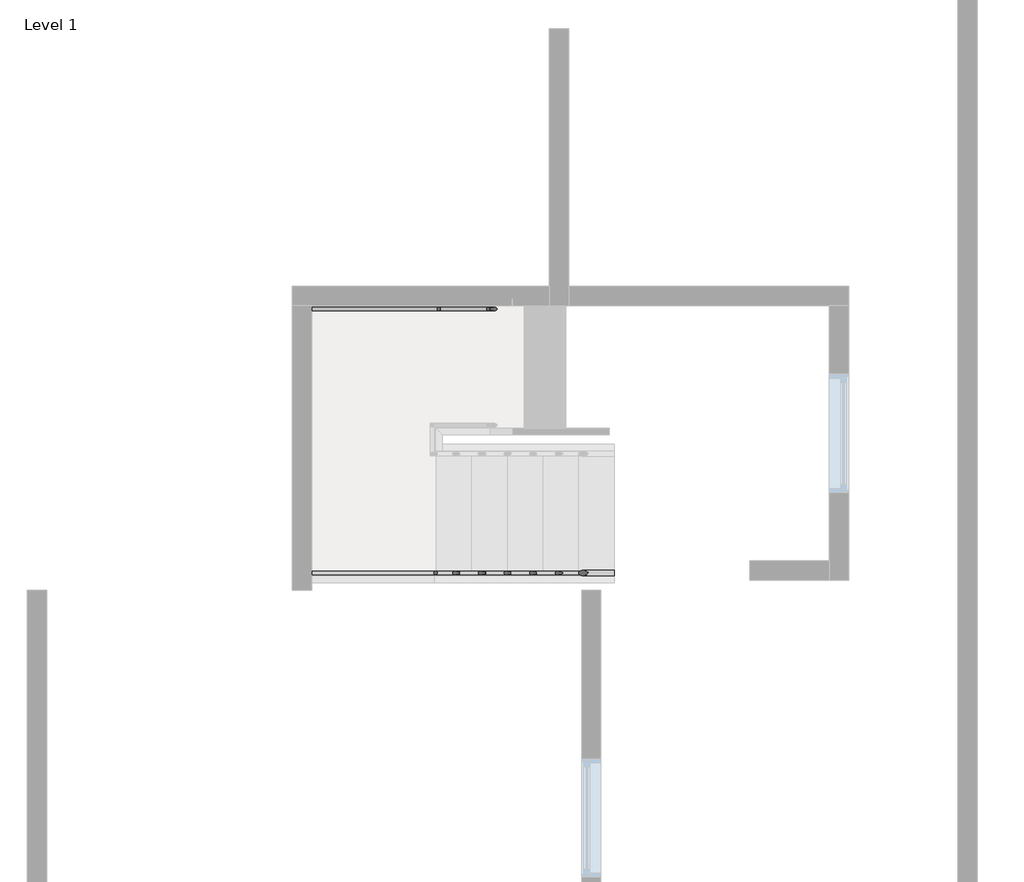
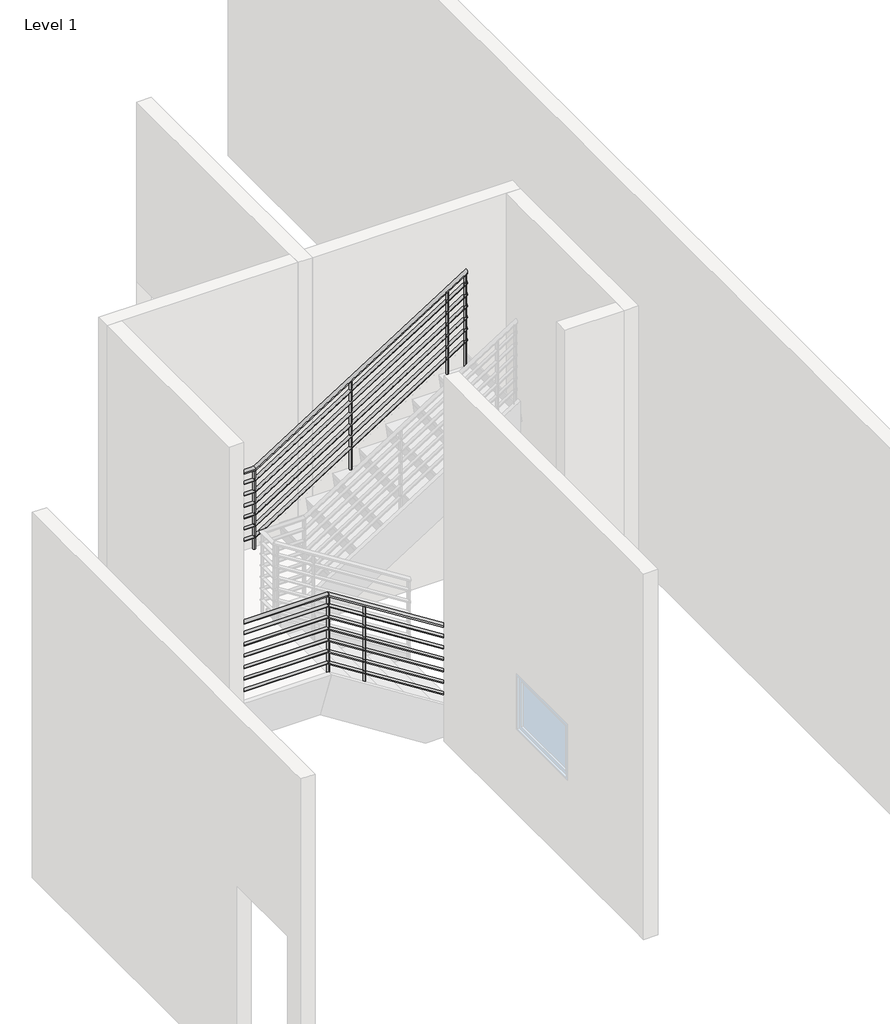
# One storey, part 2 of 4: 1 railing.
"""IFC4 building model written with IfcOpenShell, lengths in millimetres."""

from ifc_helpers import new_model, si_unit, point, frame, frame_2d, origin, place, context, project, spatial, circle_curve, ellipse_curve, trimmed, segment, composite_curve, outline, extrude, element, save
from ifc_brep_helpers import plane_surface, cylinder_surface, advanced_brep

model = new_model("IFC4")

# Units and contexts
model_context = context("Model", 3, world=origin())
ifc_project = project(units=[si_unit("LENGTHUNIT", "METRE", prefix="MILLI")], contexts=[model_context])

# Site, building, storey
site = spatial("IfcSite", under=ifc_project)
building = spatial("IfcBuilding", under=site)
storey = spatial("IfcBuildingStorey", under=building, Name="Level 1", Elevation=0.0)

# Railing
placement = place(None, origin())
element("IfcRailing", 1, ObjectType="900mm Pipe", at=placement, inside=storey, context=model_context, shape_type="SolidModel", body=[
    advanced_brep(
    [(-539.0915237, 888.4180557, 1050.2491997), (-539.0915237, 848.4180557, 1050.2491997), (-1919.8849767, 888.4180557, 1923.4782609), (-1919.8849767, 848.4180557, 1923.4782609), (-2868.717305, 888.4180557, 1923.4782609), (-2908.717305, 848.4180557, 1923.4782609), (-2868.717305, 2880.8309464, 1923.4782609), (-2908.717305, 2920.8309464, 1923.4782609), (-1501.6762623, 2880.8309464, 1923.4782609), (-1501.6762623, 2920.8309464, 1923.4782609), (692.5302847, 2880.8309464, 3311.1187649), (692.5302847, 2920.8309464, 3311.1187649)],
    [
        (0, 1, ellipse_curve(frame((-539.0915237, 868.4180557, 1050.2491997), z_axis=(1.0, 0.0, 0.0), x_axis=(0.0, 0.0, -1.0)), 23.6638438, 20.0)),
        (1, 0, ellipse_curve(frame((-539.0915237, 868.4180557, 1050.2491997), z_axis=(1.0, 0.0, 0.0), x_axis=(0.0, 0.0, -1.0)), 23.6638438, 20.0)),
        (0, 2),
        (2, 3, ellipse_curve(frame((-1919.8849767, 868.4180557, 1923.4782609), z_axis=(0.9605132043335073, 0.0, -0.2782344053149754), x_axis=(-0.278234405314975, 0.0, -0.9605132043335074)), 20.822202, 20.0)),
        (3, 1),
        (3, 2, ellipse_curve(frame((-1919.8849767, 868.4180557, 1923.4782609), z_axis=(0.9605132043335073, 0.0, -0.2782344053149754), x_axis=(-0.278234405314975, 0.0, -0.9605132043335074)), 20.822202, 20.0)),
        (2, 4),
        (4, 5, ellipse_curve(frame((-2888.717305, 868.4180557, 1923.4782609), z_axis=(0.7071067811865449, -0.7071067811865501, 0.0), x_axis=(0.7071067811865501, 0.7071067811865448, 0.0)), 28.2842712, 20.0)),
        (5, 3),
        (5, 4, ellipse_curve(frame((-2888.717305, 868.4180557, 1923.4782609), z_axis=(0.7071067811865449, -0.7071067811865501, 0.0), x_axis=(0.7071067811865501, 0.7071067811865448, 0.0)), 28.2842712, 20.0)),
        (4, 6),
        (6, 7, ellipse_curve(frame((-2888.717305, 2900.8309464, 1923.4782609), z_axis=(-0.7071067811865501, -0.7071067811865449, 0.0), x_axis=(0.7071067811865448, -0.7071067811865501, 0.0)), 28.2842712, 20.0)),
        (7, 5),
        (7, 6, ellipse_curve(frame((-2888.717305, 2900.8309464, 1923.4782609), z_axis=(-0.7071067811865501, -0.7071067811865449, 0.0), x_axis=(0.7071067811865448, -0.7071067811865501, 0.0)), 28.2842712, 20.0)),
        (6, 8),
        (8, 9, ellipse_curve(frame((-1501.6762623, 2900.8309464, 1923.4782609), z_axis=(-0.9605132043335073, 0.0, -0.27823440531497556), x_axis=(-0.2782344053149757, 0.0, 0.9605132043335073)), 20.822202, 20.0)),
        (9, 7),
        (9, 8, ellipse_curve(frame((-1501.6762623, 2900.8309464, 1923.4782609), z_axis=(-0.9605132043335073, 0.0, -0.27823440531497556), x_axis=(-0.2782344053149757, 0.0, 0.9605132043335073)), 20.822202, 20.0)),
        (10, 11, ellipse_curve(frame((692.5302847, 2900.8309464, 3311.1187649), z_axis=(1.0, 0.0, 0.0), x_axis=(0.0, 0.0, -1.0)), 23.6638438, 20.0)),
        (11, 10, ellipse_curve(frame((692.5302847, 2900.8309464, 3311.1187649), z_axis=(1.0, 0.0, 0.0), x_axis=(0.0, 0.0, -1.0)), 23.6638438, 20.0)),
        (8, 10),
        (11, 9),
    ],
    [
        plane_surface(frame((-539.0915237, 868.4180557, 1073.9130435), z_axis=(1.0, 0.0, 0.0), x_axis=(0.0, -1.0, 0.0))),
        cylinder_surface(frame((-549.7814365, 868.4180557, 1057.0096189), z_axis=(0.845171231398044, 0.0, -0.5344956404098298), x_axis=(0.0, -1.0, 0.0)), 20.0),
        cylinder_surface(frame((-1914.0915237, 868.4180557, 1923.4782609), z_axis=(1.0, 0.0, 0.0), x_axis=(0.0, -1.0, 0.0)), 20.0),
        cylinder_surface(frame((-2888.717305, 868.4180557, 1923.4782609), z_axis=(0.0, -1.0, 0.0), x_axis=(-1.0, 0.0, 0.0)), 20.0),
        cylinder_surface(frame((-2888.717305, 2900.8309464, 1923.4782609), z_axis=(-1.0, 0.0, 0.0), x_axis=(0.0, 1.0, 0.0)), 20.0),
        plane_surface(frame((692.5302847, 2900.8309464, 3334.7826087), z_axis=(1.0, 0.0, 0.0), x_axis=(0.0, 1.0, 0.0))),
        cylinder_surface(frame((-1496.7798025, 2900.8309464, 1926.5748362), z_axis=(-0.8451712313980438, 0.0, -0.5344956404098301), x_axis=(0.0, 1.0, 0.0)), 20.0),
    ],
    [
        (0, [[1, 2]]),
        (1, [[-1, 3, 4, 5]]),
        (1, [[-2, -5, 6, -3]]),
        (2, [[-4, 7, 8, 9]]),
        (2, [[-6, -9, 10, -7]]),
        (3, [[-8, 11, 12, 13]]),
        (3, [[-10, -13, 14, -11]]),
        (4, [[-12, 15, 16, 17]]),
        (4, [[-14, -17, 18, -15]]),
        (5, [[19, 20]]),
        (6, [[-16, 21, -20, 22]]),
        (6, [[-18, -22, -19, -21]]),
    ],
),
    advanced_brep(
    [(-539.0915237, 883.4180557, 931.1651606), (-539.0915237, 853.4180557, 931.1651606), (-1918.4366135, 883.4180557, 1803.4782609), (-1918.4366135, 853.4180557, 1803.4782609), (-2873.717305, 883.4180557, 1803.4782609), (-2903.717305, 853.4180557, 1803.4782609), (-2873.717305, 2885.8309464, 1803.4782609), (-2903.717305, 2915.8309464, 1803.4782609), (-1503.1246256, 2885.8309464, 1803.4782609), (-1503.1246256, 2915.8309464, 1803.4782609), (692.5302847, 2885.8309464, 3192.0347258), (692.5302847, 2915.8309464, 3192.0347258)],
    [
        (0, 1, ellipse_curve(frame((-539.0915237, 868.4180557, 931.1651606), z_axis=(1.0, 0.0, 0.0), x_axis=(0.0, 0.0, -1.0)), 17.7478828, 15.0)),
        (1, 0, ellipse_curve(frame((-539.0915237, 868.4180557, 931.1651606), z_axis=(1.0, 0.0, 0.0), x_axis=(0.0, 0.0, -1.0)), 17.7478828, 15.0)),
        (0, 2),
        (2, 3, ellipse_curve(frame((-1918.4366135, 868.4180557, 1803.4782609), z_axis=(0.9605132043335073, 0.0, -0.27823440531497545), x_axis=(-0.2782344053149749, 0.0, -0.9605132043335074)), 15.6166515, 15.0)),
        (3, 1),
        (3, 2, ellipse_curve(frame((-1918.4366135, 868.4180557, 1803.4782609), z_axis=(0.9605132043335073, 0.0, -0.27823440531497545), x_axis=(-0.2782344053149749, 0.0, -0.9605132043335074)), 15.6166515, 15.0)),
        (2, 4),
        (4, 5, ellipse_curve(frame((-2888.717305, 868.4180557, 1803.4782609), z_axis=(0.7071067811865449, -0.7071067811865501, 0.0), x_axis=(0.7071067811865501, 0.7071067811865448, 0.0)), 21.2132034, 15.0)),
        (5, 3),
        (5, 4, ellipse_curve(frame((-2888.717305, 868.4180557, 1803.4782609), z_axis=(0.7071067811865449, -0.7071067811865501, 0.0), x_axis=(0.7071067811865501, 0.7071067811865448, 0.0)), 21.2132034, 15.0)),
        (4, 6),
        (6, 7, ellipse_curve(frame((-2888.717305, 2900.8309464, 1803.4782609), z_axis=(-0.7071067811865501, -0.7071067811865449, 0.0), x_axis=(0.7071067811865448, -0.7071067811865501, 0.0)), 21.2132034, 15.0)),
        (7, 5),
        (7, 6, ellipse_curve(frame((-2888.717305, 2900.8309464, 1803.4782609), z_axis=(-0.7071067811865501, -0.7071067811865449, 0.0), x_axis=(0.7071067811865448, -0.7071067811865501, 0.0)), 21.2132034, 15.0)),
        (6, 8),
        (8, 9, ellipse_curve(frame((-1503.1246256, 2900.8309464, 1803.4782609), z_axis=(-0.9605132043335072, 0.0, -0.27823440531497556), x_axis=(-0.2782344053149761, 0.0, 0.9605132043335072)), 15.6166515, 15.0)),
        (9, 7),
        (9, 8, ellipse_curve(frame((-1503.1246256, 2900.8309464, 1803.4782609), z_axis=(-0.9605132043335072, 0.0, -0.27823440531497556), x_axis=(-0.2782344053149761, 0.0, 0.9605132043335072)), 15.6166515, 15.0)),
        (10, 11, ellipse_curve(frame((692.5302847, 2900.8309464, 3192.0347258), z_axis=(1.0, 0.0, 0.0), x_axis=(0.0, 0.0, -1.0)), 17.7478828, 15.0)),
        (11, 10, ellipse_curve(frame((692.5302847, 2900.8309464, 3192.0347258), z_axis=(1.0, 0.0, 0.0), x_axis=(0.0, 0.0, -1.0)), 17.7478828, 15.0)),
        (8, 10),
        (11, 9),
    ],
    [
        plane_surface(frame((-539.0915237, 868.4180557, 948.9130435), z_axis=(1.0, 0.0, 0.0), x_axis=(0.0, -1.0, 0.0))),
        cylinder_surface(frame((-547.1089583, 868.4180557, 936.235475), z_axis=(0.845171231398044, 0.0, -0.5344956404098299), x_axis=(0.0, -1.0, 0.0)), 15.0),
        cylinder_surface(frame((-1914.0915237, 868.4180557, 1803.4782609), z_axis=(1.0, 0.0, 0.0), x_axis=(0.0, -1.0, 0.0)), 15.0),
        cylinder_surface(frame((-2888.717305, 868.4180557, 1803.4782609), z_axis=(0.0, -1.0, 0.0), x_axis=(-1.0, 0.0, 0.0)), 15.0),
        cylinder_surface(frame((-2888.717305, 2900.8309464, 1803.4782609), z_axis=(-1.0, 0.0, 0.0), x_axis=(0.0, 1.0, 0.0)), 15.0),
        plane_surface(frame((692.5302847, 2900.8309464, 3209.7826087), z_axis=(1.0, 0.0, 0.0), x_axis=(0.0, 1.0, 0.0))),
        cylinder_surface(frame((-1499.4522807, 2900.8309464, 1805.8006924), z_axis=(-0.8451712313980437, 0.0, -0.5344956404098301), x_axis=(0.0, 1.0, 0.0)), 15.0),
    ],
    [
        (0, [[1, 2]]),
        (1, [[-1, 3, 4, 5]]),
        (1, [[-2, -5, 6, -3]]),
        (2, [[-4, 7, 8, 9]]),
        (2, [[-6, -9, 10, -7]]),
        (3, [[-8, 11, 12, 13]]),
        (3, [[-10, -13, 14, -11]]),
        (4, [[-12, 15, 16, 17]]),
        (4, [[-14, -17, 18, -15]]),
        (5, [[19, 20]]),
        (6, [[-16, 21, -20, 22]]),
        (6, [[-18, -22, -19, -21]]),
    ],
),
    advanced_brep(
    [(-539.0915237, 883.4180557, 806.1651606), (-539.0915237, 853.4180557, 806.1651606), (-1918.4366135, 883.4180557, 1678.4782609), (-1918.4366135, 853.4180557, 1678.4782609), (-2873.717305, 883.4180557, 1678.4782609), (-2903.717305, 853.4180557, 1678.4782609), (-2873.717305, 2885.8309464, 1678.4782609), (-2903.717305, 2915.8309464, 1678.4782609), (-1503.1246256, 2885.8309464, 1678.4782609), (-1503.1246256, 2915.8309464, 1678.4782609), (692.5302847, 2885.8309464, 3067.0347258), (692.5302847, 2915.8309464, 3067.0347258)],
    [
        (0, 1, ellipse_curve(frame((-539.0915237, 868.4180557, 806.1651606), z_axis=(1.0, 0.0, 0.0), x_axis=(0.0, 0.0, -1.0)), 17.7478828, 15.0)),
        (1, 0, ellipse_curve(frame((-539.0915237, 868.4180557, 806.1651606), z_axis=(1.0, 0.0, 0.0), x_axis=(0.0, 0.0, -1.0)), 17.7478828, 15.0)),
        (0, 2),
        (2, 3, ellipse_curve(frame((-1918.4366135, 868.4180557, 1678.4782609), z_axis=(0.9605132043335073, 0.0, -0.27823440531497545), x_axis=(-0.2782344053149749, 0.0, -0.9605132043335074)), 15.6166515, 15.0)),
        (3, 1),
        (3, 2, ellipse_curve(frame((-1918.4366135, 868.4180557, 1678.4782609), z_axis=(0.9605132043335073, 0.0, -0.27823440531497545), x_axis=(-0.2782344053149749, 0.0, -0.9605132043335074)), 15.6166515, 15.0)),
        (2, 4),
        (4, 5, ellipse_curve(frame((-2888.717305, 868.4180557, 1678.4782609), z_axis=(0.7071067811865449, -0.7071067811865501, 0.0), x_axis=(0.7071067811865501, 0.7071067811865448, 0.0)), 21.2132034, 15.0)),
        (5, 3),
        (5, 4, ellipse_curve(frame((-2888.717305, 868.4180557, 1678.4782609), z_axis=(0.7071067811865449, -0.7071067811865501, 0.0), x_axis=(0.7071067811865501, 0.7071067811865448, 0.0)), 21.2132034, 15.0)),
        (4, 6),
        (6, 7, ellipse_curve(frame((-2888.717305, 2900.8309464, 1678.4782609), z_axis=(-0.7071067811865501, -0.7071067811865449, 0.0), x_axis=(0.7071067811865448, -0.7071067811865501, 0.0)), 21.2132034, 15.0)),
        (7, 5),
        (7, 6, ellipse_curve(frame((-2888.717305, 2900.8309464, 1678.4782609), z_axis=(-0.7071067811865501, -0.7071067811865449, 0.0), x_axis=(0.7071067811865448, -0.7071067811865501, 0.0)), 21.2132034, 15.0)),
        (6, 8),
        (8, 9, ellipse_curve(frame((-1503.1246256, 2900.8309464, 1678.4782609), z_axis=(-0.9605132043335073, 0.0, -0.27823440531497556), x_axis=(-0.27823440531497573, 0.0, 0.9605132043335072)), 15.6166515, 15.0)),
        (9, 7),
        (9, 8, ellipse_curve(frame((-1503.1246256, 2900.8309464, 1678.4782609), z_axis=(-0.9605132043335073, 0.0, -0.27823440531497556), x_axis=(-0.27823440531497573, 0.0, 0.9605132043335072)), 15.6166515, 15.0)),
        (10, 11, ellipse_curve(frame((692.5302847, 2900.8309464, 3067.0347258), z_axis=(1.0, 0.0, 0.0), x_axis=(0.0, 0.0, -1.0)), 17.7478828, 15.0)),
        (11, 10, ellipse_curve(frame((692.5302847, 2900.8309464, 3067.0347258), z_axis=(1.0, 0.0, 0.0), x_axis=(0.0, 0.0, -1.0)), 17.7478828, 15.0)),
        (8, 10),
        (11, 9),
    ],
    [
        plane_surface(frame((-539.0915237, 868.4180557, 823.9130435), z_axis=(1.0, 0.0, 0.0), x_axis=(0.0, -1.0, 0.0))),
        cylinder_surface(frame((-547.1089583, 868.4180557, 811.235475), z_axis=(0.845171231398044, 0.0, -0.5344956404098299), x_axis=(0.0, -1.0, 0.0)), 15.0),
        cylinder_surface(frame((-1914.0915237, 868.4180557, 1678.4782609), z_axis=(1.0, 0.0, 0.0), x_axis=(0.0, -1.0, 0.0)), 15.0),
        cylinder_surface(frame((-2888.717305, 868.4180557, 1678.4782609), z_axis=(0.0, -1.0, 0.0), x_axis=(-1.0, 0.0, 0.0)), 15.0),
        cylinder_surface(frame((-2888.717305, 2900.8309464, 1678.4782609), z_axis=(-1.0, 0.0, 0.0), x_axis=(0.0, 1.0, 0.0)), 15.0),
        plane_surface(frame((692.5302847, 2900.8309464, 3084.7826087), z_axis=(1.0, 0.0, 0.0), x_axis=(0.0, 1.0, 0.0))),
        cylinder_surface(frame((-1499.4522807, 2900.8309464, 1680.8006924), z_axis=(-0.8451712313980438, 0.0, -0.5344956404098301), x_axis=(0.0, 1.0, 0.0)), 15.0),
    ],
    [
        (0, [[1, 2]]),
        (1, [[-1, 3, 4, 5]]),
        (1, [[-2, -5, 6, -3]]),
        (2, [[-4, 7, 8, 9]]),
        (2, [[-6, -9, 10, -7]]),
        (3, [[-8, 11, 12, 13]]),
        (3, [[-10, -13, 14, -11]]),
        (4, [[-12, 15, 16, 17]]),
        (4, [[-14, -17, 18, -15]]),
        (5, [[19, 20]]),
        (6, [[-16, 21, -20, 22]]),
        (6, [[-18, -22, -19, -21]]),
    ],
),
    advanced_brep(
    [(-539.0915237, 883.4180557, 681.1651606), (-539.0915237, 853.4180557, 681.1651606), (-1918.4366135, 883.4180557, 1553.4782609), (-1918.4366135, 853.4180557, 1553.4782609), (-2873.717305, 883.4180557, 1553.4782609), (-2903.717305, 853.4180557, 1553.4782609), (-2873.717305, 2885.8309464, 1553.4782609), (-2903.717305, 2915.8309464, 1553.4782609), (-1503.1246256, 2885.8309464, 1553.4782609), (-1503.1246256, 2915.8309464, 1553.4782609), (692.5302847, 2885.8309464, 2942.0347258), (692.5302847, 2915.8309464, 2942.0347258)],
    [
        (0, 1, ellipse_curve(frame((-539.0915237, 868.4180557, 681.1651606), z_axis=(1.0, 0.0, 0.0), x_axis=(0.0, 0.0, -1.0)), 17.7478828, 15.0)),
        (1, 0, ellipse_curve(frame((-539.0915237, 868.4180557, 681.1651606), z_axis=(1.0, 0.0, 0.0), x_axis=(0.0, 0.0, -1.0)), 17.7478828, 15.0)),
        (0, 2),
        (2, 3, ellipse_curve(frame((-1918.4366135, 868.4180557, 1553.4782609), z_axis=(0.9605132043335073, 0.0, -0.27823440531497545), x_axis=(-0.2782344053149749, 0.0, -0.9605132043335074)), 15.6166515, 15.0)),
        (3, 1),
        (3, 2, ellipse_curve(frame((-1918.4366135, 868.4180557, 1553.4782609), z_axis=(0.9605132043335073, 0.0, -0.27823440531497545), x_axis=(-0.2782344053149749, 0.0, -0.9605132043335074)), 15.6166515, 15.0)),
        (2, 4),
        (4, 5, ellipse_curve(frame((-2888.717305, 868.4180557, 1553.4782609), z_axis=(0.7071067811865449, -0.7071067811865501, 0.0), x_axis=(0.7071067811865501, 0.7071067811865448, 0.0)), 21.2132034, 15.0)),
        (5, 3),
        (5, 4, ellipse_curve(frame((-2888.717305, 868.4180557, 1553.4782609), z_axis=(0.7071067811865449, -0.7071067811865501, 0.0), x_axis=(0.7071067811865501, 0.7071067811865448, 0.0)), 21.2132034, 15.0)),
        (4, 6),
        (6, 7, ellipse_curve(frame((-2888.717305, 2900.8309464, 1553.4782609), z_axis=(-0.7071067811865501, -0.7071067811865449, 0.0), x_axis=(0.7071067811865448, -0.7071067811865501, 0.0)), 21.2132034, 15.0)),
        (7, 5),
        (7, 6, ellipse_curve(frame((-2888.717305, 2900.8309464, 1553.4782609), z_axis=(-0.7071067811865501, -0.7071067811865449, 0.0), x_axis=(0.7071067811865448, -0.7071067811865501, 0.0)), 21.2132034, 15.0)),
        (6, 8),
        (8, 9, ellipse_curve(frame((-1503.1246256, 2900.8309464, 1553.4782609), z_axis=(-0.9605132043335073, 0.0, -0.27823440531497556), x_axis=(-0.27823440531497573, 0.0, 0.9605132043335072)), 15.6166515, 15.0)),
        (9, 7),
        (9, 8, ellipse_curve(frame((-1503.1246256, 2900.8309464, 1553.4782609), z_axis=(-0.9605132043335073, 0.0, -0.27823440531497556), x_axis=(-0.27823440531497573, 0.0, 0.9605132043335072)), 15.6166515, 15.0)),
        (10, 11, ellipse_curve(frame((692.5302847, 2900.8309464, 2942.0347258), z_axis=(1.0, 0.0, 0.0), x_axis=(0.0, 0.0, -1.0)), 17.7478828, 15.0)),
        (11, 10, ellipse_curve(frame((692.5302847, 2900.8309464, 2942.0347258), z_axis=(1.0, 0.0, 0.0), x_axis=(0.0, 0.0, -1.0)), 17.7478828, 15.0)),
        (8, 10),
        (11, 9),
    ],
    [
        plane_surface(frame((-539.0915237, 868.4180557, 698.9130435), z_axis=(1.0, 0.0, 0.0), x_axis=(0.0, -1.0, 0.0))),
        cylinder_surface(frame((-547.1089583, 868.4180557, 686.235475), z_axis=(0.845171231398044, 0.0, -0.5344956404098299), x_axis=(0.0, -1.0, 0.0)), 15.0),
        cylinder_surface(frame((-1914.0915237, 868.4180557, 1553.4782609), z_axis=(1.0, 0.0, 0.0), x_axis=(0.0, -1.0, 0.0)), 15.0),
        cylinder_surface(frame((-2888.717305, 868.4180557, 1553.4782609), z_axis=(0.0, -1.0, 0.0), x_axis=(-1.0, 0.0, 0.0)), 15.0),
        cylinder_surface(frame((-2888.717305, 2900.8309464, 1553.4782609), z_axis=(-1.0, 0.0, 0.0), x_axis=(0.0, 1.0, 0.0)), 15.0),
        plane_surface(frame((692.5302847, 2900.8309464, 2959.7826087), z_axis=(1.0, 0.0, 0.0), x_axis=(0.0, 1.0, 0.0))),
        cylinder_surface(frame((-1499.4522807, 2900.8309464, 1555.8006924), z_axis=(-0.8451712313980438, 0.0, -0.5344956404098301), x_axis=(0.0, 1.0, 0.0)), 15.0),
    ],
    [
        (0, [[1, 2]]),
        (1, [[-1, 3, 4, 5]]),
        (1, [[-2, -5, 6, -3]]),
        (2, [[-4, 7, 8, 9]]),
        (2, [[-6, -9, 10, -7]]),
        (3, [[-8, 11, 12, 13]]),
        (3, [[-10, -13, 14, -11]]),
        (4, [[-12, 15, 16, 17]]),
        (4, [[-14, -17, 18, -15]]),
        (5, [[19, 20]]),
        (6, [[-16, 21, -20, 22]]),
        (6, [[-18, -22, -19, -21]]),
    ],
),
    advanced_brep(
    [(-539.0915237, 883.4180557, 556.1651606), (-539.0915237, 853.4180557, 556.1651606), (-1918.4366135, 883.4180557, 1428.4782609), (-1918.4366135, 853.4180557, 1428.4782609), (-2873.717305, 883.4180557, 1428.4782609), (-2903.717305, 853.4180557, 1428.4782609), (-2873.717305, 2885.8309464, 1428.4782609), (-2903.717305, 2915.8309464, 1428.4782609), (-1503.1246256, 2885.8309464, 1428.4782609), (-1503.1246256, 2915.8309464, 1428.4782609), (692.5302847, 2885.8309464, 2817.0347258), (692.5302847, 2915.8309464, 2817.0347258)],
    [
        (0, 1, ellipse_curve(frame((-539.0915237, 868.4180557, 556.1651606), z_axis=(1.0, 0.0, 0.0), x_axis=(0.0, 0.0, -1.0)), 17.7478828, 15.0)),
        (1, 0, ellipse_curve(frame((-539.0915237, 868.4180557, 556.1651606), z_axis=(1.0, 0.0, 0.0), x_axis=(0.0, 0.0, -1.0)), 17.7478828, 15.0)),
        (0, 2),
        (2, 3, ellipse_curve(frame((-1918.4366135, 868.4180557, 1428.4782609), z_axis=(0.9605132043335073, 0.0, -0.27823440531497545), x_axis=(-0.2782344053149749, 0.0, -0.9605132043335074)), 15.6166515, 15.0)),
        (3, 1),
        (3, 2, ellipse_curve(frame((-1918.4366135, 868.4180557, 1428.4782609), z_axis=(0.9605132043335073, 0.0, -0.27823440531497545), x_axis=(-0.2782344053149749, 0.0, -0.9605132043335074)), 15.6166515, 15.0)),
        (2, 4),
        (4, 5, ellipse_curve(frame((-2888.717305, 868.4180557, 1428.4782609), z_axis=(0.7071067811865449, -0.7071067811865501, 0.0), x_axis=(0.7071067811865501, 0.7071067811865448, 0.0)), 21.2132034, 15.0)),
        (5, 3),
        (5, 4, ellipse_curve(frame((-2888.717305, 868.4180557, 1428.4782609), z_axis=(0.7071067811865449, -0.7071067811865501, 0.0), x_axis=(0.7071067811865501, 0.7071067811865448, 0.0)), 21.2132034, 15.0)),
        (4, 6),
        (6, 7, ellipse_curve(frame((-2888.717305, 2900.8309464, 1428.4782609), z_axis=(-0.7071067811865501, -0.7071067811865449, 0.0), x_axis=(0.7071067811865448, -0.7071067811865501, 0.0)), 21.2132034, 15.0)),
        (7, 5),
        (7, 6, ellipse_curve(frame((-2888.717305, 2900.8309464, 1428.4782609), z_axis=(-0.7071067811865501, -0.7071067811865449, 0.0), x_axis=(0.7071067811865448, -0.7071067811865501, 0.0)), 21.2132034, 15.0)),
        (6, 8),
        (8, 9, ellipse_curve(frame((-1503.1246256, 2900.8309464, 1428.4782609), z_axis=(-0.9605132043335073, 0.0, -0.27823440531497556), x_axis=(-0.27823440531497573, 0.0, 0.9605132043335072)), 15.6166515, 15.0)),
        (9, 7),
        (9, 8, ellipse_curve(frame((-1503.1246256, 2900.8309464, 1428.4782609), z_axis=(-0.9605132043335073, 0.0, -0.27823440531497556), x_axis=(-0.27823440531497573, 0.0, 0.9605132043335072)), 15.6166515, 15.0)),
        (10, 11, ellipse_curve(frame((692.5302847, 2900.8309464, 2817.0347258), z_axis=(1.0, 0.0, 0.0), x_axis=(0.0, 0.0, -1.0)), 17.7478828, 15.0)),
        (11, 10, ellipse_curve(frame((692.5302847, 2900.8309464, 2817.0347258), z_axis=(1.0, 0.0, 0.0), x_axis=(0.0, 0.0, -1.0)), 17.7478828, 15.0)),
        (8, 10),
        (11, 9),
    ],
    [
        plane_surface(frame((-539.0915237, 868.4180557, 573.9130435), z_axis=(1.0, 0.0, 0.0), x_axis=(0.0, -1.0, 0.0))),
        cylinder_surface(frame((-547.1089583, 868.4180557, 561.235475), z_axis=(0.845171231398044, 0.0, -0.5344956404098299), x_axis=(0.0, -1.0, 0.0)), 15.0),
        cylinder_surface(frame((-1914.0915237, 868.4180557, 1428.4782609), z_axis=(1.0, 0.0, 0.0), x_axis=(0.0, -1.0, 0.0)), 15.0),
        cylinder_surface(frame((-2888.717305, 868.4180557, 1428.4782609), z_axis=(0.0, -1.0, 0.0), x_axis=(-1.0, 0.0, 0.0)), 15.0),
        cylinder_surface(frame((-2888.717305, 2900.8309464, 1428.4782609), z_axis=(-1.0, 0.0, 0.0), x_axis=(0.0, 1.0, 0.0)), 15.0),
        plane_surface(frame((692.5302847, 2900.8309464, 2834.7826087), z_axis=(1.0, 0.0, 0.0), x_axis=(0.0, 1.0, 0.0))),
        cylinder_surface(frame((-1499.4522807, 2900.8309464, 1430.8006924), z_axis=(-0.8451712313980438, 0.0, -0.5344956404098301), x_axis=(0.0, 1.0, 0.0)), 15.0),
    ],
    [
        (0, [[1, 2]]),
        (1, [[-1, 3, 4, 5]]),
        (1, [[-2, -5, 6, -3]]),
        (2, [[-4, 7, 8, 9]]),
        (2, [[-6, -9, 10, -7]]),
        (3, [[-8, 11, 12, 13]]),
        (3, [[-10, -13, 14, -11]]),
        (4, [[-12, 15, 16, 17]]),
        (4, [[-14, -17, 18, -15]]),
        (5, [[19, 20]]),
        (6, [[-16, 21, -20, 22]]),
        (6, [[-18, -22, -19, -21]]),
    ],
),
    advanced_brep(
    [(-539.0915237, 883.4180557, 431.1651606), (-539.0915237, 853.4180557, 431.1651606), (-1918.4366135, 883.4180557, 1303.4782609), (-1918.4366135, 853.4180557, 1303.4782609), (-2873.717305, 883.4180557, 1303.4782609), (-2903.717305, 853.4180557, 1303.4782609), (-2873.717305, 2885.8309464, 1303.4782609), (-2903.717305, 2915.8309464, 1303.4782609), (-1503.1246256, 2885.8309464, 1303.4782609), (-1503.1246256, 2915.8309464, 1303.4782609), (692.5302847, 2885.8309464, 2692.0347258), (692.5302847, 2915.8309464, 2692.0347258)],
    [
        (0, 1, ellipse_curve(frame((-539.0915237, 868.4180557, 431.1651606), z_axis=(1.0, 0.0, 0.0), x_axis=(0.0, 0.0, -1.0)), 17.7478828, 15.0)),
        (1, 0, ellipse_curve(frame((-539.0915237, 868.4180557, 431.1651606), z_axis=(1.0, 0.0, 0.0), x_axis=(0.0, 0.0, -1.0)), 17.7478828, 15.0)),
        (0, 2),
        (2, 3, ellipse_curve(frame((-1918.4366135, 868.4180557, 1303.4782609), z_axis=(0.9605132043335073, 0.0, -0.27823440531497545), x_axis=(-0.2782344053149749, 0.0, -0.9605132043335074)), 15.6166515, 15.0)),
        (3, 1),
        (3, 2, ellipse_curve(frame((-1918.4366135, 868.4180557, 1303.4782609), z_axis=(0.9605132043335073, 0.0, -0.27823440531497545), x_axis=(-0.2782344053149749, 0.0, -0.9605132043335074)), 15.6166515, 15.0)),
        (2, 4),
        (4, 5, ellipse_curve(frame((-2888.717305, 868.4180557, 1303.4782609), z_axis=(0.7071067811865449, -0.7071067811865501, 0.0), x_axis=(0.7071067811865501, 0.7071067811865448, 0.0)), 21.2132034, 15.0)),
        (5, 3),
        (5, 4, ellipse_curve(frame((-2888.717305, 868.4180557, 1303.4782609), z_axis=(0.7071067811865449, -0.7071067811865501, 0.0), x_axis=(0.7071067811865501, 0.7071067811865448, 0.0)), 21.2132034, 15.0)),
        (4, 6),
        (6, 7, ellipse_curve(frame((-2888.717305, 2900.8309464, 1303.4782609), z_axis=(-0.7071067811865501, -0.7071067811865449, 0.0), x_axis=(0.7071067811865448, -0.7071067811865501, 0.0)), 21.2132034, 15.0)),
        (7, 5),
        (7, 6, ellipse_curve(frame((-2888.717305, 2900.8309464, 1303.4782609), z_axis=(-0.7071067811865501, -0.7071067811865449, 0.0), x_axis=(0.7071067811865448, -0.7071067811865501, 0.0)), 21.2132034, 15.0)),
        (6, 8),
        (8, 9, ellipse_curve(frame((-1503.1246256, 2900.8309464, 1303.4782609), z_axis=(-0.9605132043335072, 0.0, -0.27823440531497556), x_axis=(-0.2782344053149761, 0.0, 0.9605132043335072)), 15.6166515, 15.0)),
        (9, 7),
        (9, 8, ellipse_curve(frame((-1503.1246256, 2900.8309464, 1303.4782609), z_axis=(-0.9605132043335072, 0.0, -0.27823440531497556), x_axis=(-0.2782344053149761, 0.0, 0.9605132043335072)), 15.6166515, 15.0)),
        (10, 11, ellipse_curve(frame((692.5302847, 2900.8309464, 2692.0347258), z_axis=(1.0, 0.0, 0.0), x_axis=(0.0, 0.0, -1.0)), 17.7478828, 15.0)),
        (11, 10, ellipse_curve(frame((692.5302847, 2900.8309464, 2692.0347258), z_axis=(1.0, 0.0, 0.0), x_axis=(0.0, 0.0, -1.0)), 17.7478828, 15.0)),
        (8, 10),
        (11, 9),
    ],
    [
        plane_surface(frame((-539.0915237, 868.4180557, 448.9130435), z_axis=(1.0, 0.0, 0.0), x_axis=(0.0, -1.0, 0.0))),
        cylinder_surface(frame((-547.1089583, 868.4180557, 436.235475), z_axis=(0.845171231398044, 0.0, -0.5344956404098299), x_axis=(0.0, -1.0, 0.0)), 15.0),
        cylinder_surface(frame((-1914.0915237, 868.4180557, 1303.4782609), z_axis=(1.0, 0.0, 0.0), x_axis=(0.0, -1.0, 0.0)), 15.0),
        cylinder_surface(frame((-2888.717305, 868.4180557, 1303.4782609), z_axis=(0.0, -1.0, 0.0), x_axis=(-1.0, 0.0, 0.0)), 15.0),
        cylinder_surface(frame((-2888.717305, 2900.8309464, 1303.4782609), z_axis=(-1.0, 0.0, 0.0), x_axis=(0.0, 1.0, 0.0)), 15.0),
        plane_surface(frame((692.5302847, 2900.8309464, 2709.7826087), z_axis=(1.0, 0.0, 0.0), x_axis=(0.0, 1.0, 0.0))),
        cylinder_surface(frame((-1499.4522807, 2900.8309464, 1305.8006924), z_axis=(-0.8451712313980437, 0.0, -0.5344956404098301), x_axis=(0.0, 1.0, 0.0)), 15.0),
    ],
    [
        (0, [[1, 2]]),
        (1, [[-1, 3, 4, 5]]),
        (1, [[-2, -5, 6, -3]]),
        (2, [[-4, 7, 8, 9]]),
        (2, [[-6, -9, 10, -7]]),
        (3, [[-8, 11, 12, 13]]),
        (3, [[-10, -13, 14, -11]]),
        (4, [[-12, 15, 16, 17]]),
        (4, [[-14, -17, 18, -15]]),
        (5, [[19, 20]]),
        (6, [[-16, 21, -20, 22]]),
        (6, [[-18, -22, -19, -21]]),
    ],
),
    advanced_brep(
    [(-539.0915237, 883.4180557, 306.1651606), (-539.0915237, 853.4180557, 306.1651606), (-1918.4366135, 883.4180557, 1178.4782609), (-1918.4366135, 853.4180557, 1178.4782609), (-2873.717305, 883.4180557, 1178.4782609), (-2903.717305, 853.4180557, 1178.4782609), (-2873.717305, 2885.8309464, 1178.4782609), (-2903.717305, 2915.8309464, 1178.4782609), (-1503.1246256, 2885.8309464, 1178.4782609), (-1503.1246256, 2915.8309464, 1178.4782609), (692.5302847, 2885.8309464, 2567.0347258), (692.5302847, 2915.8309464, 2567.0347258)],
    [
        (0, 1, ellipse_curve(frame((-539.0915237, 868.4180557, 306.1651606), z_axis=(1.0, 0.0, 0.0), x_axis=(0.0, 0.0, -1.0)), 17.7478828, 15.0)),
        (1, 0, ellipse_curve(frame((-539.0915237, 868.4180557, 306.1651606), z_axis=(1.0, 0.0, 0.0), x_axis=(0.0, 0.0, -1.0)), 17.7478828, 15.0)),
        (0, 2),
        (2, 3, ellipse_curve(frame((-1918.4366135, 868.4180557, 1178.4782609), z_axis=(0.9605132043335073, 0.0, -0.27823440531497545), x_axis=(-0.2782344053149749, 0.0, -0.9605132043335074)), 15.6166515, 15.0)),
        (3, 1),
        (3, 2, ellipse_curve(frame((-1918.4366135, 868.4180557, 1178.4782609), z_axis=(0.9605132043335073, 0.0, -0.27823440531497545), x_axis=(-0.2782344053149749, 0.0, -0.9605132043335074)), 15.6166515, 15.0)),
        (2, 4),
        (4, 5, ellipse_curve(frame((-2888.717305, 868.4180557, 1178.4782609), z_axis=(0.7071067811865449, -0.7071067811865501, 0.0), x_axis=(0.7071067811865501, 0.7071067811865448, 0.0)), 21.2132034, 15.0)),
        (5, 3),
        (5, 4, ellipse_curve(frame((-2888.717305, 868.4180557, 1178.4782609), z_axis=(0.7071067811865449, -0.7071067811865501, 0.0), x_axis=(0.7071067811865501, 0.7071067811865448, 0.0)), 21.2132034, 15.0)),
        (4, 6),
        (6, 7, ellipse_curve(frame((-2888.717305, 2900.8309464, 1178.4782609), z_axis=(-0.7071067811865501, -0.7071067811865449, 0.0), x_axis=(0.7071067811865448, -0.7071067811865501, 0.0)), 21.2132034, 15.0)),
        (7, 5),
        (7, 6, ellipse_curve(frame((-2888.717305, 2900.8309464, 1178.4782609), z_axis=(-0.7071067811865501, -0.7071067811865449, 0.0), x_axis=(0.7071067811865448, -0.7071067811865501, 0.0)), 21.2132034, 15.0)),
        (6, 8),
        (8, 9, ellipse_curve(frame((-1503.1246256, 2900.8309464, 1178.4782609), z_axis=(-0.9605132043335073, 0.0, -0.27823440531497556), x_axis=(-0.27823440531497573, 0.0, 0.9605132043335072)), 15.6166515, 15.0)),
        (9, 7),
        (9, 8, ellipse_curve(frame((-1503.1246256, 2900.8309464, 1178.4782609), z_axis=(-0.9605132043335073, 0.0, -0.27823440531497556), x_axis=(-0.27823440531497573, 0.0, 0.9605132043335072)), 15.6166515, 15.0)),
        (10, 11, ellipse_curve(frame((692.5302847, 2900.8309464, 2567.0347258), z_axis=(1.0, 0.0, 0.0), x_axis=(0.0, 0.0, -1.0)), 17.7478828, 15.0)),
        (11, 10, ellipse_curve(frame((692.5302847, 2900.8309464, 2567.0347258), z_axis=(1.0, 0.0, 0.0), x_axis=(0.0, 0.0, -1.0)), 17.7478828, 15.0)),
        (8, 10),
        (11, 9),
    ],
    [
        plane_surface(frame((-539.0915237, 868.4180557, 323.9130435), z_axis=(1.0, 0.0, 0.0), x_axis=(0.0, -1.0, 0.0))),
        cylinder_surface(frame((-547.1089583, 868.4180557, 311.235475), z_axis=(0.845171231398044, 0.0, -0.5344956404098299), x_axis=(0.0, -1.0, 0.0)), 15.0),
        cylinder_surface(frame((-1914.0915237, 868.4180557, 1178.4782609), z_axis=(1.0, 0.0, 0.0), x_axis=(0.0, -1.0, 0.0)), 15.0),
        cylinder_surface(frame((-2888.717305, 868.4180557, 1178.4782609), z_axis=(0.0, -1.0, 0.0), x_axis=(-1.0, 0.0, 0.0)), 15.0),
        cylinder_surface(frame((-2888.717305, 2900.8309464, 1178.4782609), z_axis=(-1.0, 0.0, 0.0), x_axis=(0.0, 1.0, 0.0)), 15.0),
        plane_surface(frame((692.5302847, 2900.8309464, 2584.7826087), z_axis=(1.0, 0.0, 0.0), x_axis=(0.0, 1.0, 0.0))),
        cylinder_surface(frame((-1499.4522807, 2900.8309464, 1180.8006924), z_axis=(-0.8451712313980438, 0.0, -0.5344956404098301), x_axis=(0.0, 1.0, 0.0)), 15.0),
    ],
    [
        (0, [[1, 2]]),
        (1, [[-1, 3, 4, 5]]),
        (1, [[-2, -5, 6, -3]]),
        (2, [[-4, 7, 8, 9]]),
        (2, [[-6, -9, 10, -7]]),
        (3, [[-8, 11, 12, 13]]),
        (3, [[-10, -13, 14, -11]]),
        (4, [[-12, 15, 16, 17]]),
        (4, [[-14, -17, 18, -15]]),
        (5, [[19, 20]]),
        (6, [[-16, 21, -20, 22]]),
        (6, [[-18, -22, -19, -21]]),
    ],
),
    advanced_brep(
    [(492.5302847, 2913.3309464, 3160.9727077), (492.5302847, 2888.3309464, 3160.9727077), (492.5302847, 2888.3309464, 2260.8695652), (492.5302847, 2913.3309464, 2260.8695652)],
    [
        (0, 1, ellipse_curve(frame((492.5302847, 2900.8309464, 3160.9727077), z_axis=(0.5344956404098302, 0.0, -0.8451712313980437), x_axis=(0.8451712313980437, 0.0, 0.53449564040983)), 14.7899024, 12.5)),
        (1, 2),
        (2, 3, circle_curve(frame((492.5302847, 2900.8309464, 2260.8695652), z_axis=(0.0, 0.0, 1.0), x_axis=(0.0, -1.0, 0.0)), 12.5)),
        (3, 0),
        (3, 2, circle_curve(frame((492.5302847, 2900.8309464, 2260.8695652), z_axis=(0.0, 0.0, 1.0), x_axis=(0.0, -1.0, 0.0)), 12.5)),
        (1, 0, ellipse_curve(frame((492.5302847, 2900.8309464, 3160.9727077), z_axis=(0.5344956404098302, 0.0, -0.8451712313980437), x_axis=(0.8451712313980437, 0.0, 0.53449564040983)), 14.7899024, 12.5)),
    ],
    [
        cylinder_surface(frame((492.5302847, 2900.8309464, 2160.8695652), z_axis=(0.0, 0.0, 1.0), x_axis=(0.0, -1.0, 0.0)), 12.5),
        plane_surface(frame((517.5302847, 2875.8309464, 3176.7829843), z_axis=(-0.5344956404098302, 0.0, 0.8451712313980437), x_axis=(0.0, 1.0, 0.0))),
        plane_surface(frame((467.5302847, 2875.8309464, 2260.8695652), z_axis=(0.0, 0.0, -1.0), x_axis=(0.0, 1.0, 0.0))),
    ],
    [
        (0, [[1, 2, 3, 4]]),
        (0, [[5, -2, 6, -4]]),
        (1, [[-6, -1]]),
        (2, [[-5, -3]]),
    ],
),
    advanced_brep(
    [(-507.4697153, 2913.3309464, 2528.5616405), (-507.4697153, 2888.3309464, 2528.5616405), (-507.4697153, 2888.3309464, 1565.2173913), (-507.4697153, 2913.3309464, 1565.2173913)],
    [
        (0, 1, ellipse_curve(frame((-507.4697153, 2900.8309464, 2528.5616405), z_axis=(0.5344956404098302, 0.0, -0.8451712313980437), x_axis=(0.8451712313980437, 0.0, 0.53449564040983)), 14.7899024, 12.5)),
        (1, 2),
        (2, 3, circle_curve(frame((-507.4697153, 2900.8309464, 1565.2173913), z_axis=(0.0, 0.0, 1.0), x_axis=(0.0, -1.0, 0.0)), 12.5)),
        (3, 0),
        (3, 2, circle_curve(frame((-507.4697153, 2900.8309464, 1565.2173913), z_axis=(0.0, 0.0, 1.0), x_axis=(0.0, -1.0, 0.0)), 12.5)),
        (1, 0, ellipse_curve(frame((-507.4697153, 2900.8309464, 2528.5616405), z_axis=(0.5344956404098302, 0.0, -0.8451712313980437), x_axis=(0.8451712313980437, 0.0, 0.53449564040983)), 14.7899024, 12.5)),
    ],
    [
        cylinder_surface(frame((-507.4697153, 2900.8309464, 1465.2173913), z_axis=(0.0, 0.0, 1.0), x_axis=(0.0, -1.0, 0.0)), 12.5),
        plane_surface(frame((-482.4697153, 2875.8309464, 2544.3719172), z_axis=(-0.5344956404098302, 0.0, 0.8451712313980437), x_axis=(0.0, 1.0, 0.0))),
        plane_surface(frame((-532.4697153, 2875.8309464, 1565.2173913), z_axis=(0.0, 0.0, -1.0), x_axis=(0.0, 1.0, 0.0))),
    ],
    [
        (0, [[1, 2, 3, 4]]),
        (0, [[5, -2, 6, -4]]),
        (1, [[-6, -1]]),
        (2, [[-5, -3]]),
    ],
),
    extrude(outline(composite_curve([segment(trimmed(circle_curve(frame_2d((-1888.717305, 2900.8309464)), 12.5), [point((-1888.717305, 2888.3309464))], [point((-1888.717305, 2913.3309464))], False, "CARTESIAN"), True, "CONTINUOUS"), segment(trimmed(circle_curve(frame_2d((-1888.717305, 2900.8309464)), 12.5), [point((-1888.717305, 2913.3309464))], [point((-1888.717305, 2888.3309464))], False, "CARTESIAN"), True, "CONTINUOUS")], self_intersect=False)), frame((0.0, 0.0, 1043.4782609), z_axis=(0.0, 0.0, 1.0), x_axis=(1.0, 0.0, 0.0)), (0.0, 0.0, 1.0), 860.0),
    extrude(outline(composite_curve([segment(trimmed(circle_curve(frame_2d((-2888.717305, 2868.4180557)), 12.5), [point((-2876.217305, 2868.4180557))], [point((-2901.217305, 2868.4180557))], False, "CARTESIAN"), True, "CONTINUOUS"), segment(trimmed(circle_curve(frame_2d((-2888.717305, 2868.4180557)), 12.5), [point((-2901.217305, 2868.4180557))], [point((-2876.217305, 2868.4180557))], False, "CARTESIAN"), True, "CONTINUOUS")], self_intersect=False)), frame((0.0, 0.0, 1043.4782609), z_axis=(0.0, 0.0, 1.0), x_axis=(1.0, 0.0, 0.0)), (0.0, 0.0, 1.0), 860.0),
    extrude(outline(composite_curve([segment(trimmed(circle_curve(frame_2d((-2888.717305, 1868.4180557)), 12.5), [point((-2876.217305, 1868.4180557))], [point((-2901.217305, 1868.4180557))], False, "CARTESIAN"), True, "CONTINUOUS"), segment(trimmed(circle_curve(frame_2d((-2888.717305, 1868.4180557)), 12.5), [point((-2901.217305, 1868.4180557))], [point((-2876.217305, 1868.4180557))], False, "CARTESIAN"), True, "CONTINUOUS")], self_intersect=False)), frame((0.0, 0.0, 1043.4782609), z_axis=(0.0, 0.0, 1.0), x_axis=(1.0, 0.0, 0.0)), (0.0, 0.0, 1.0), 860.0),
    advanced_brep(
    [(-1539.0915237, 855.9180557, 1658.9964231), (-1539.0915237, 880.9180557, 1658.9964231), (-1539.0915237, 880.9180557, 695.6521739), (-1539.0915237, 855.9180557, 695.6521739)],
    [
        (0, 1, ellipse_curve(frame((-1539.0915237, 868.4180557, 1658.9964231), z_axis=(-0.5344956404098302, 0.0, -0.8451712313980437), x_axis=(-0.8451712313980437, 0.0, 0.53449564040983)), 14.7899024, 12.5)),
        (1, 2),
        (2, 3, circle_curve(frame((-1539.0915237, 868.4180557, 695.6521739), z_axis=(0.0, 0.0, 1.0), x_axis=(0.0, 1.0, 0.0)), 12.5)),
        (3, 0),
        (3, 2, circle_curve(frame((-1539.0915237, 868.4180557, 695.6521739), z_axis=(0.0, 0.0, 1.0), x_axis=(0.0, 1.0, 0.0)), 12.5)),
        (1, 0, ellipse_curve(frame((-1539.0915237, 868.4180557, 1658.9964231), z_axis=(-0.5344956404098302, 0.0, -0.8451712313980437), x_axis=(-0.8451712313980437, 0.0, 0.53449564040983)), 14.7899024, 12.5)),
    ],
    [
        cylinder_surface(frame((-1539.0915237, 868.4180557, 595.6521739), z_axis=(0.0, 0.0, 1.0), x_axis=(0.0, 1.0, 0.0)), 12.5),
        plane_surface(frame((-1564.0915237, 893.4180557, 1674.8066998), z_axis=(0.5344956404098302, 0.0, 0.8451712313980437), x_axis=(0.0, -1.0, 0.0))),
        plane_surface(frame((-1514.0915237, 893.4180557, 695.6521739), z_axis=(0.0, 0.0, -1.0), x_axis=(0.0, -1.0, 0.0))),
    ],
    [
        (0, [[1, 2, 3, 4]]),
        (0, [[5, -2, 6, -4]]),
        (1, [[-6, -1]]),
        (2, [[-5, -3]]),
    ],
),
    extrude(outline(composite_curve([segment(trimmed(circle_curve(frame_2d((-1507.4697153, 2900.8309464)), 12.5), [point((-1507.4697153, 2888.3309464))], [point((-1507.4697153, 2913.3309464))], False, "CARTESIAN"), True, "CONTINUOUS"), segment(trimmed(circle_curve(frame_2d((-1507.4697153, 2900.8309464)), 12.5), [point((-1507.4697153, 2913.3309464))], [point((-1507.4697153, 2888.3309464))], False, "CARTESIAN"), True, "CONTINUOUS")], self_intersect=False)), frame((0.0, 0.0, 1043.4782609), z_axis=(0.0, 0.0, 1.0), x_axis=(1.0, 0.0, 0.0)), (0.0, 0.0, 1.0), 860.0),
    extrude(outline(composite_curve([segment(trimmed(circle_curve(frame_2d((-2888.717305, 2900.8309464)), 12.5), [point((-2876.217305, 2900.8309464))], [point((-2901.217305, 2900.8309464))], False, "CARTESIAN"), True, "CONTINUOUS"), segment(trimmed(circle_curve(frame_2d((-2888.717305, 2900.8309464)), 12.5), [point((-2901.217305, 2900.8309464))], [point((-2876.217305, 2900.8309464))], False, "CARTESIAN"), True, "CONTINUOUS")], self_intersect=False)), frame((0.0, 0.0, 1043.4782609), z_axis=(0.0, 0.0, 1.0), x_axis=(1.0, 0.0, 0.0)), (0.0, 0.0, 1.0), 860.0),
    extrude(outline(composite_curve([segment(trimmed(circle_curve(frame_2d((-2888.717305, 868.4180557)), 12.5), [point((-2888.717305, 880.9180557))], [point((-2888.717305, 855.9180557))], False, "CARTESIAN"), True, "CONTINUOUS"), segment(trimmed(circle_curve(frame_2d((-2888.717305, 868.4180557)), 12.5), [point((-2888.717305, 855.9180557))], [point((-2888.717305, 880.9180557))], False, "CARTESIAN"), True, "CONTINUOUS")], self_intersect=False)), frame((0.0, 0.0, 1043.4782609), z_axis=(0.0, 0.0, 1.0), x_axis=(1.0, 0.0, 0.0)), (0.0, 0.0, 1.0), 860.0),
    extrude(outline(composite_curve([segment(trimmed(circle_curve(frame_2d((-1914.0915237, 868.4180557)), 12.5), [point((-1914.0915237, 880.9180557))], [point((-1914.0915237, 855.9180557))], False, "CARTESIAN"), True, "CONTINUOUS"), segment(trimmed(circle_curve(frame_2d((-1914.0915237, 868.4180557)), 12.5), [point((-1914.0915237, 855.9180557))], [point((-1914.0915237, 880.9180557))], False, "CARTESIAN"), True, "CONTINUOUS")], self_intersect=False)), frame((0.0, 0.0, 1043.4782609), z_axis=(0.0, 0.0, 1.0), x_axis=(1.0, 0.0, 0.0)), (0.0, 0.0, 1.0), 860.0),
    advanced_brep(
    [(680.0302847, 2913.3309464, 3279.5497828), (680.0302847, 2888.3309464, 3279.5497828), (680.0302847, 2888.3309464, 2260.8695652), (680.0302847, 2913.3309464, 2260.8695652)],
    [
        (0, 1, ellipse_curve(frame((680.0302847, 2900.8309464, 3279.5497828), z_axis=(0.5344956404098286, 0.0, -0.8451712313980447), x_axis=(0.8451712313980447, 0.0, 0.5344956404098286)), 14.7899024, 12.5)),
        (1, 2),
        (2, 3, circle_curve(frame((680.0302847, 2900.8309464, 2260.8695652), z_axis=(0.0, 0.0, 1.0), x_axis=(0.0, -1.0, 0.0)), 12.5)),
        (3, 0),
        (3, 2, circle_curve(frame((680.0302847, 2900.8309464, 2260.8695652), z_axis=(0.0, 0.0, 1.0), x_axis=(0.0, -1.0, 0.0)), 12.5)),
        (1, 0, ellipse_curve(frame((680.0302847, 2900.8309464, 3279.5497828), z_axis=(0.5344956404098286, 0.0, -0.8451712313980447), x_axis=(0.8451712313980447, 0.0, 0.5344956404098286)), 14.7899024, 12.5)),
    ],
    [
        cylinder_surface(frame((680.0302847, 2900.8309464, 2160.8695652), z_axis=(0.0, 0.0, 1.0), x_axis=(0.0, -1.0, 0.0)), 12.5),
        plane_surface(frame((705.0302847, 2875.8309464, 3295.3600594), z_axis=(-0.5344956404098286, 0.0, 0.8451712313980447), x_axis=(0.0, 1.0, 0.0))),
        plane_surface(frame((655.0302847, 2875.8309464, 2260.8695652), z_axis=(0.0, 0.0, -1.0), x_axis=(0.0, 1.0, 0.0))),
    ],
    [
        (0, [[1, 2, 3, 4]]),
        (0, [[5, -2, 6, -4]]),
        (1, [[-6, -1]]),
        (2, [[-5, -3]]),
    ],
),
    advanced_brep(
    [(-551.5915237, 855.9180557, 1034.4904942), (-551.5915237, 880.9180557, 1034.4904942), (-551.5915237, 880.9180557, 173.9130435), (-551.5915237, 855.9180557, 173.9130435)],
    [
        (0, 1, ellipse_curve(frame((-551.5915237, 868.4180557, 1034.4904942), z_axis=(-0.5344956404098302, 0.0, -0.8451712313980437), x_axis=(-0.8451712313980437, 0.0, 0.53449564040983)), 14.7899024, 12.5)),
        (1, 2),
        (2, 3, circle_curve(frame((-551.5915237, 868.4180557, 173.9130435), z_axis=(0.0, 0.0, 1.0), x_axis=(0.0, 1.0, 0.0)), 12.5)),
        (3, 0),
        (3, 2, circle_curve(frame((-551.5915237, 868.4180557, 173.9130435), z_axis=(0.0, 0.0, 1.0), x_axis=(0.0, 1.0, 0.0)), 12.5)),
        (1, 0, ellipse_curve(frame((-551.5915237, 868.4180557, 1034.4904942), z_axis=(-0.5344956404098302, 0.0, -0.8451712313980437), x_axis=(-0.8451712313980437, 0.0, 0.53449564040983)), 14.7899024, 12.5)),
    ],
    [
        cylinder_surface(frame((-551.5915237, 868.4180557, 73.9130435), z_axis=(0.0, 0.0, 1.0), x_axis=(0.0, 1.0, 0.0)), 12.5),
        plane_surface(frame((-576.5915237, 893.4180557, 1050.3007709), z_axis=(0.5344956404098302, 0.0, 0.8451712313980437), x_axis=(0.0, -1.0, 0.0))),
        plane_surface(frame((-526.5915237, 893.4180557, 173.9130435), z_axis=(0.0, 0.0, -1.0), x_axis=(0.0, -1.0, 0.0))),
    ],
    [
        (0, [[1, 2, 3, 4]]),
        (0, [[5, -2, 6, -4]]),
        (1, [[-6, -1]]),
        (2, [[-5, -3]]),
    ],
),
])

save(model, "model.ifc")

# Revit data of these elements
# Type "900mm Pipe"
#   built-in parameter 1008612 = 0.019685 (stored number, unit not read)
#   built-in parameter 1008611 = 0.0984252 (stored number, unit not read)
#   built-in parameter 1008609 = 6.56168 (stored number, unit not read)
#   built-in parameter 1008604 = 0.19685 (stored number, unit not read)
#   built-in parameter 1008603 = 0.164042 (stored number, unit not read)
#   Railing Height = 900 mm
#   built-in parameter 1008630 = 2
#   built-in parameter 1008610 = 2
#   built-in parameter 1008605 = 1
#   built-in parameter 1008618 = M_Baluster - Round : 25mm
# Element 1 (IfcRailing, "900mm Pipe")
#   Phase Created = New Construction
